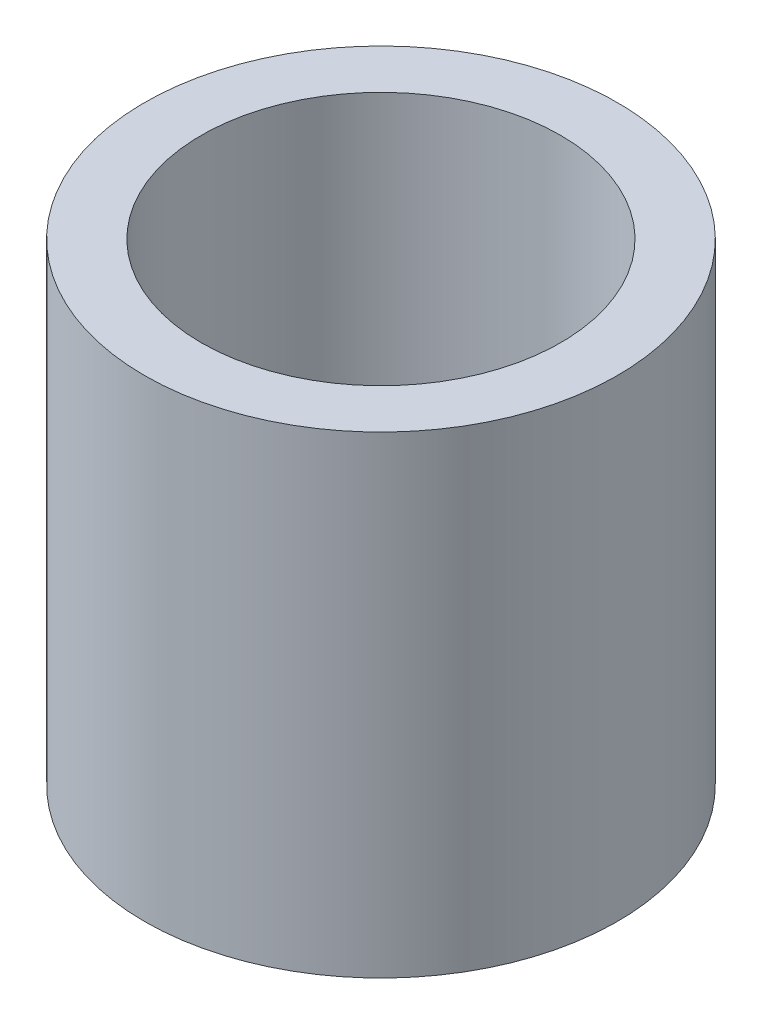
ISO-10303-21;
HEADER;
FILE_DESCRIPTION(('STEP AP214'),'2;1');
FILE_NAME('part.step','',(''),(''),'','','');
FILE_SCHEMA(('AUTOMOTIVE_DESIGN { 1 0 10303 214 1 1 1 1 }'));
ENDSEC;
DATA;
#1=APPLICATION_CONTEXT('core data for automotive mechanical design processes');
#2=APPLICATION_PROTOCOL_DEFINITION('international standard','automotive_design',2000,#1);
#3=PRODUCT_CONTEXT('',#1,'mechanical');
#4=PRODUCT('Part','Part','',(#3));
#5=PRODUCT_RELATED_PRODUCT_CATEGORY('part','',(#4));
#6=PRODUCT_DEFINITION_FORMATION('','',#4);
#7=PRODUCT_DEFINITION_CONTEXT('part definition',#1,'design');
#8=PRODUCT_DEFINITION('design','',#6,#7);
#9=PRODUCT_DEFINITION_SHAPE('','',#8);
#10=(LENGTH_UNIT() NAMED_UNIT(*) SI_UNIT(.MILLI.,.METRE.));
#11=(NAMED_UNIT(*) PLANE_ANGLE_UNIT() SI_UNIT($,.RADIAN.));
#12=(NAMED_UNIT(*) SI_UNIT($,.STERADIAN.) SOLID_ANGLE_UNIT());
#13=UNCERTAINTY_MEASURE_WITH_UNIT(LENGTH_MEASURE(1.E-05),#10,'distance_accuracy_value','');
#14=(GEOMETRIC_REPRESENTATION_CONTEXT(3) GLOBAL_UNCERTAINTY_ASSIGNED_CONTEXT((#13)) GLOBAL_UNIT_ASSIGNED_CONTEXT((#10,
#11,#12)) REPRESENTATION_CONTEXT('',''));
#15=CARTESIAN_POINT('',(0.,0.,0.));
#16=DIRECTION('',(0.,0.,1.));
#17=DIRECTION('',(1.,0.,0.));
#18=AXIS2_PLACEMENT_3D('',#15,#16,#17);
#19=CARTESIAN_POINT('',(0.,25.,0.));
#20=DIRECTION('',(0.,1.,0.));
#21=DIRECTION('',(0.,0.,1.));
#22=AXIS2_PLACEMENT_3D('',#19,#20,#21);
#23=PLANE('',#22);
#24=CARTESIAN_POINT('',(0.,25.,0.));
#25=DIRECTION('',(0.,1.,0.));
#26=DIRECTION('',(0.,0.,1.));
#27=AXIS2_PLACEMENT_3D('',#24,#25,#26);
#28=CIRCLE('',#27,12.5);
#29=CARTESIAN_POINT('',(0.,25.,12.5));
#30=VERTEX_POINT('',#29);
#31=EDGE_CURVE('E10',#30,#30,#28,.T.);
#32=ORIENTED_EDGE('',*,*,#31,.T.);
#33=EDGE_LOOP('',(#32));
#34=FACE_BOUND('',#33,.T.);
#35=CARTESIAN_POINT('',(0.,25.,0.));
#36=DIRECTION('',(0.,1.,0.));
#37=DIRECTION('',(0.,0.,1.));
#38=AXIS2_PLACEMENT_3D('',#35,#36,#37);
#39=CIRCLE('',#38,9.5);
#40=CARTESIAN_POINT('',(0.,25.,9.5));
#41=VERTEX_POINT('',#40);
#42=EDGE_CURVE('E49',#41,#41,#39,.T.);
#43=ORIENTED_EDGE('',*,*,#42,.F.);
#44=EDGE_LOOP('',(#43));
#45=FACE_BOUND('',#44,.T.);
#46=ADVANCED_FACE('F39',(#34,#45),#23,.T.);
#47=CARTESIAN_POINT('',(0.,0.,0.));
#48=DIRECTION('',(0.,1.,0.));
#49=DIRECTION('',(0.,0.,1.));
#50=AXIS2_PLACEMENT_3D('',#47,#48,#49);
#51=PLANE('',#50);
#52=CARTESIAN_POINT('',(0.,0.,0.));
#53=DIRECTION('',(0.,1.,0.));
#54=DIRECTION('',(0.,0.,1.));
#55=AXIS2_PLACEMENT_3D('',#52,#53,#54);
#56=CIRCLE('',#55,12.5);
#57=CARTESIAN_POINT('',(0.,0.,12.5));
#58=VERTEX_POINT('',#57);
#59=EDGE_CURVE('E43',#58,#58,#56,.T.);
#60=ORIENTED_EDGE('',*,*,#59,.F.);
#61=EDGE_LOOP('',(#60));
#62=FACE_BOUND('',#61,.T.);
#63=CARTESIAN_POINT('',(0.,0.,0.));
#64=DIRECTION('',(0.,1.,0.));
#65=DIRECTION('',(0.,0.,1.));
#66=AXIS2_PLACEMENT_3D('',#63,#64,#65);
#67=CIRCLE('',#66,9.5);
#68=CARTESIAN_POINT('',(0.,0.,9.5));
#69=VERTEX_POINT('',#68);
#70=EDGE_CURVE('E55',#69,#69,#67,.T.);
#71=ORIENTED_EDGE('',*,*,#70,.T.);
#72=EDGE_LOOP('',(#71));
#73=FACE_BOUND('',#72,.T.);
#74=ADVANCED_FACE('F65',(#62,#73),#51,.F.);
#75=CARTESIAN_POINT('',(0.,25.,0.));
#76=DIRECTION('',(0.,-1.,0.));
#77=DIRECTION('',(0.,0.,-1.));
#78=AXIS2_PLACEMENT_3D('',#75,#76,#77);
#79=CYLINDRICAL_SURFACE('',#78,12.5);
#80=ORIENTED_EDGE('',*,*,#31,.F.);
#81=EDGE_LOOP('',(#80));
#82=FACE_BOUND('',#81,.T.);
#83=ORIENTED_EDGE('',*,*,#59,.T.);
#84=EDGE_LOOP('',(#83));
#85=FACE_BOUND('',#84,.T.);
#86=ADVANCED_FACE('F41',(#82,#85),#79,.T.);
#87=CARTESIAN_POINT('',(0.,25.,0.));
#88=DIRECTION('',(0.,-1.,0.));
#89=DIRECTION('',(0.,0.,-1.));
#90=AXIS2_PLACEMENT_3D('',#87,#88,#89);
#91=CYLINDRICAL_SURFACE('',#90,9.5);
#92=ORIENTED_EDGE('',*,*,#42,.T.);
#93=EDGE_LOOP('',(#92));
#94=FACE_BOUND('',#93,.T.);
#95=ORIENTED_EDGE('',*,*,#70,.F.);
#96=EDGE_LOOP('',(#95));
#97=FACE_BOUND('',#96,.T.);
#98=ADVANCED_FACE('F59',(#94,#97),#91,.F.);
#99=CLOSED_SHELL('',(#46,#74,#86,#98));
#100=MANIFOLD_SOLID_BREP('B2',#99);
#101=ADVANCED_BREP_SHAPE_REPRESENTATION('',(#18,#100),#14);
#102=SHAPE_DEFINITION_REPRESENTATION(#9,#101);
ENDSEC;
END-ISO-10303-21;
